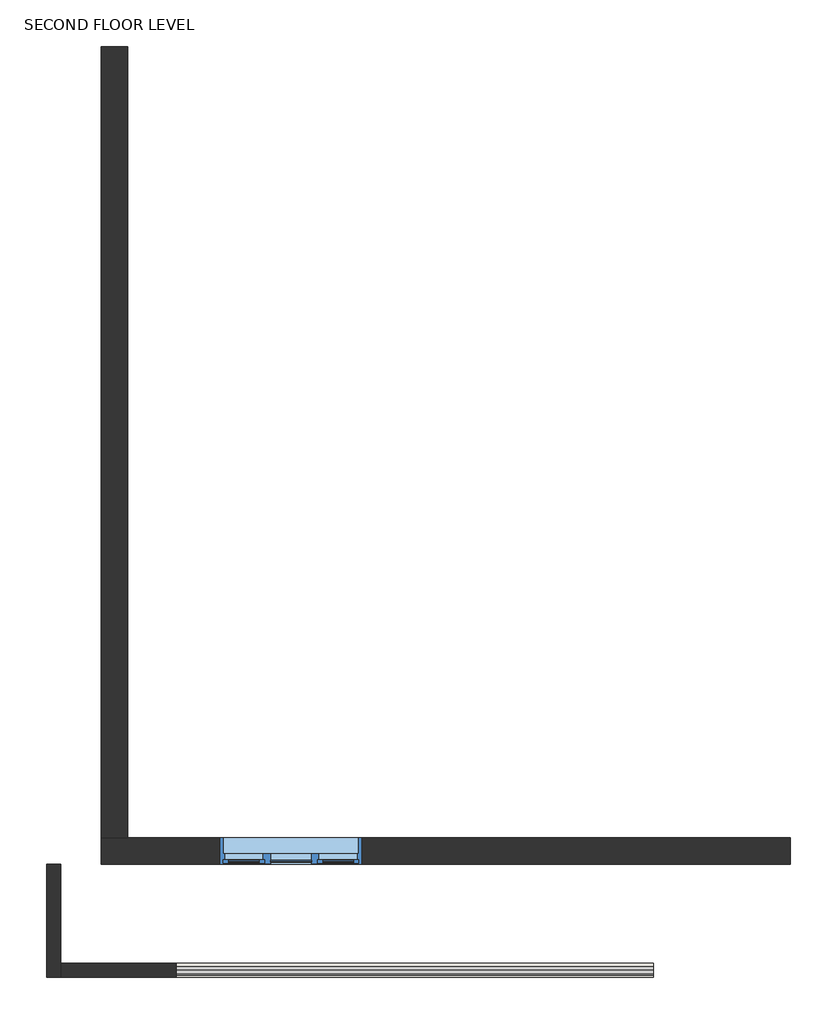
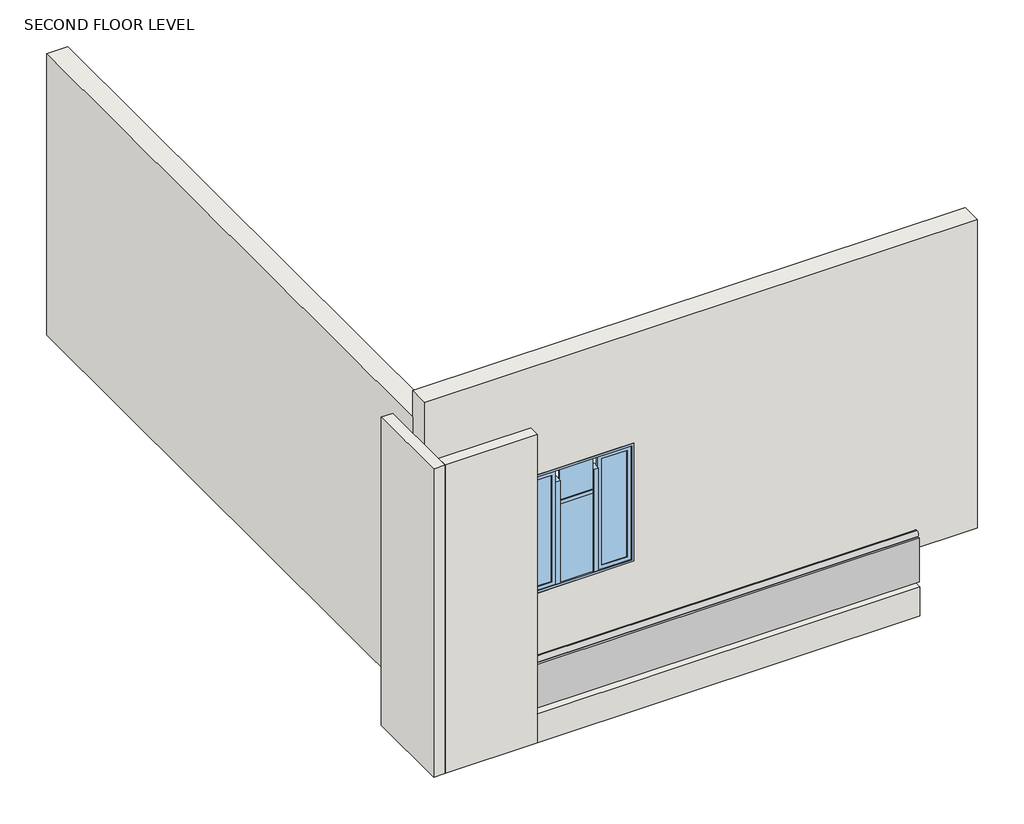
# One storey, incomplete: 5 walls, 1 member, 1 plate, 1 window.
"""IFC4 building model written with IfcOpenShell, lengths in millimetres."""

from ifc_helpers import new_model, si_unit, frame, origin, place, context, project, spatial, polyline, outline, extrude, faceted_brep, transform, mapped, element, save
from components import member_62657261, system_panel_glazed_289ab79d, window_273a115f

model = new_model("IFC4")

# Units and contexts
model_context = context("Model", 3, world=origin())
ifc_project = project(units=[si_unit("LENGTHUNIT", "METRE", prefix="MILLI")], contexts=[model_context])

# Site, building, storey
site = spatial("IfcSite", under=ifc_project)
building = spatial("IfcBuilding", under=site)
storey = spatial("IfcBuildingStorey", under=building, Name="SECOND FLOOR LEVEL", Elevation=7924.8)

# Member
placement = place(None, origin())
member_shape = member_62657261(model_context)
element("IfcMember", 1, ObjectType="Circular Mullion : 2.5\" Circular", at=placement, inside=storey, context=model_context, shape_type="MappedRepresentation", body=[
    mapped(member_shape, transform((7881.4271331, -12888.5768494, 8864.6), x_axis=(0.0, 0.0, 1.0), y_axis=(0.0, -1.0, 0.0), z_axis=(1.0, 0.0, 0.0))),
])

# Plate
system_panel_glazed_shape = system_panel_glazed_289ab79d(model_context)
element("IfcPlate", 2, ObjectType="System Panel : Glazed", at=placement, inside=storey, context=model_context, shape_type="MappedRepresentation", body=[
    mapped(system_panel_glazed_shape, transform((5824.0271331, -12888.5768494, 8305.8), x_axis=(1.0, 0.0, 0.0), y_axis=(0.0, 1.0, 0.0), z_axis=(0.0, 0.0, 1.0))),
])

# Walls
element("IfcWall", 3, ObjectType="9\"", at=placement, inside=storey, context=model_context, shape_type="Brep", body=[
    faceted_brep([(3118.9271331, -11975.7643494, 7924.8), (9062.5271331, -11975.7643494, 7924.8), (9062.5271331, -11975.7643494, 11430.0), (3118.9271331, -11975.7643494, 11430.0), (4147.6271331, -11975.7643494, 10185.4), (5366.8271331, -11975.7643494, 10185.4), (5366.8271331, -11975.7643494, 8839.2), (4147.6271331, -11975.7643494, 8839.2), (3118.9271331, -11747.1643494, 7924.8), (3118.9271331, -11747.1643494, 11127.6170633), (3118.9271331, -11747.1643494, 11430.0), (9062.5271331, -11747.1643494, 11430.0), (9062.5271331, -11747.1643494, 7924.8), (3347.5271331, -11747.1643494, 7924.8), (4147.6271331, -11747.1643494, 10185.4), (4147.6271331, -11747.1643494, 8839.2), (5366.8271331, -11747.1643494, 8839.2), (5366.8271331, -11747.1643494, 10185.4)], [[[0, 1, 2, 3], [4, 5, 6, 7]], [[8, 9, 10, 11, 12, 13], [14, 15, 16, 17]], [[1, 0, 8, 13, 12]], [[2, 1, 12, 11]], [[3, 2, 11, 10]], [[15, 14, 4, 7]], [[16, 15, 7, 6]], [[17, 16, 6, 5]], [[14, 17, 5, 4]], [[0, 3, 10, 9, 8]]]),
])
element("IfcWall", 4, ObjectType="9\"", at=placement, inside=storey, context=model_context, shape_type="SweptSolid", body=[
    extrude(outline(polyline([(3347.5271331, -4927.2643494), (3347.5271331, -11747.1643494), (3118.9271331, -11747.1643494), (3118.9271331, -4927.2643494), (3347.5271331, -4927.2643494)])), frame((0.0, 0.0, 7924.8), z_axis=(0.0, 0.0, 1.0), x_axis=(1.0, 0.0, 0.0)), (0.0, 0.0, 1.0), 3202.8170633),
])
element("IfcWall", 5, ObjectType="Interior - 4 7/8\" Partition (1-hr)", at=placement, inside=storey, context=model_context, shape_type="SweptSolid", body=[
    extrude(outline(polyline([(3766.6271331, -12826.6643494), (7881.4271331, -12826.6643494), (7881.4271331, -12950.4893494), (3766.6271331, -12950.4893494), (3766.6271331, -12826.6643494)])), frame((0.0, 0.0, 7924.8), z_axis=(0.0, 0.0, 1.0), x_axis=(1.0, 0.0, 0.0)), (0.0, 0.0, 1.0), 330.2),
])
element("IfcWall", 6, ObjectType="Interior - 4 7/8\" Partition (1-hr)", at=placement, inside=storey, context=model_context, shape_type="Brep", body=[
    faceted_brep([(2649.0271331, -11975.7643494, 7924.8), (2649.0271331, -12950.4893494, 7924.8), (2649.0271331, -12950.4893494, 11430.0), (2649.0271331, -11975.7643494, 11430.0), (2772.8521331, -11975.7643494, 7924.8), (2772.8521331, -11975.7643494, 11430.0), (2772.8521331, -12826.6643494, 11430.0), (2772.8521331, -12950.4893494, 11430.0), (2772.8521331, -12950.4893494, 7924.8), (2772.8521331, -12826.6643494, 7924.8)], [[[0, 1, 2, 3]], [[4, 5, 6, 7, 8, 9]], [[1, 0, 4, 9, 8]], [[3, 2, 7, 6, 5]], [[0, 3, 5, 4]], [[2, 1, 8, 7]]]),
])
element("IfcWall", 7, ObjectType="Interior - 4 7/8\" Partition (1-hr)", at=placement, inside=storey, context=model_context, shape_type="Brep", body=[
    faceted_brep([(3766.6271331, -12826.6643494, 7924.8), (2772.8521331, -12826.6643494, 7924.8), (2772.8521331, -12826.6643494, 11430.0), (3766.6271331, -12826.6643494, 11430.0), (3766.6271331, -12826.6643494, 8255.0), (3766.6271331, -12950.4893494, 7924.8), (3766.6271331, -12950.4893494, 8255.0), (3766.6271331, -12950.4893494, 11430.0), (2772.8521331, -12950.4893494, 11430.0), (2772.8521331, -12950.4893494, 7924.8)], [[[0, 1, 2, 3, 4]], [[5, 6, 7, 8, 9]], [[1, 0, 5, 9]], [[3, 2, 8, 7]], [[0, 4, 3, 7, 6, 5]], [[2, 1, 9, 8]]]),
])

# Window
window_shape = window_273a115f(model_context)
element("IfcWindow", 8, ObjectType="Window-Casement-Triple-Middle-Transom : 48\" x 53\"", at=placement, inside=storey, context=model_context, shape_type="MappedRepresentation", body=[
    mapped(window_shape, transform((4757.2271331, -11861.4643494, 7924.8), x_axis=(-1.0, 0.0, 0.0), y_axis=(0.0, -1.0, 0.0), z_axis=(0.0, 0.0, 1.0))),
])

save(model, "model.ifc")

# Revit data of these elements
# Type "Circular Mullion : 2.5\" Circular"
#   built-in parameter 1007350 = 0.104167 (stored number, unit not read)
# Type "System Panel : Glazed"
#   Construction Type Id = "GSP4R"
#   Analytic Construction = "1/8 in Pilkington single glazing"
#   Visual Light Transmittance = 0.9
#   Solar Heat Gain Coefficient = 0.86
#   Heat Transfer Coefficient (U) = 1.18115 BTU/(h·ft²·°F)
#   Define Thermal Properties by = 1
# Type "9\""
#   Assembly Code = "B2010"
#   Layers, outside or top first: 0' - 9" no material (function 1)
# Type "Interior - 4 7/8\" Partition (1-hr)"
#   Assembly Code = "C1010145"
#   Layers, outside or top first: 0' - 0 5/8" "Gypsum Wall Board" (function 5); 0' - 3 5/8" "Metal Stud Layer" (function 1); 0' - 0 5/8" "Gypsum Wall Board" (function 5)
# Type "Window-Casement-Triple-Middle-Transom : 48\" x 53\""
#   Type Mark = "18"
#   Fire Rating = "0.5h"
#   Assembly Code = "B2020100"
#   Analytic Construction = "Double glazing - domestic"
#   Window Width = 1' - 4"
#   Window Inset [instance default] = 0' - 0 5/8"
#   Wall Thickness [instance default] = 0' - 6"
#   Visual Light Transmittance = 0.81
#   Transom Height Ratio = 0.3
#   Thermal Resistance (R) = 1.8146 (h·ft²·°F)/BTU
#   Solar Heat Gain Coefficient = 0.76
#   Rough Width = 4' - 0 1/2"
#   Rough Height = 4' - 5 1/2"
#   Heat Transfer Coefficient (U) = 0.5511 BTU/(h·ft²·°F)
#   Height = 4' - 5"
#   Transom Height = 1' - 3.9"
#   Frame Gap 3 [instance default] = 0' - 1 83/128"
#   Frame Gap 2 [instance default] = 0' - 0 5/8"
#   Frame Gap 1 = 0' - 1 51/128"
#   Default Sill Height = 3' - 0"
#   Width = 4' - 0"
#   Frame Material = Metal - Aluminum
#   Glass Panel Material = Glass
#   Wall Closure = (empty or 0)
# Element 1 (IfcMember, "Circular Mullion : 2.5\" Circular")
#   Phase Created = New Construction
#   Materials on its faces: "Aluminum"
# Element 2 (IfcPlate, "System Panel : Glazed")
#   Phase Created = New Construction
#   Materials on its faces: "Glass"
# Element 3 (IfcWall, "9\"")
#   Top Offset = 0' - 0"
#   Base Offset = 0' - 0"
#   wall height = 11' - 6"
#   Phase Created = New Construction
#   Base Constraint = SECOND FLOOR LEVEL
#   Top Constraint = ROOF LEVEL
#   Materials on its faces: "Default Wall"
# Element 4 (IfcWall, "9\"")
#   Top Offset = 0' - 0"
#   Base Offset = 0' - 0"
#   Unconnected Height = 10' - 6.09516"
#   wall height = 10' - 6.09516"
#   Phase Created = New Construction
#   Base Constraint = SECOND FLOOR LEVEL
#   Materials on its faces: "Default Wall"
# Element 5 (IfcWall, "Interior - 4 7/8\" Partition (1-hr)")
#   Top Offset = 0' - 0"
#   Base Offset = 0' - 0"
#   Unconnected Height = 1' - 1"
#   wall height = 1' - 1"
#   Phase Created = New Construction
#   Base Constraint = SECOND FLOOR LEVEL
#   Materials on its faces: "Default Wall", "Gypsum Wall Board"
# Element 6 (IfcWall, "Interior - 4 7/8\" Partition (1-hr)")
#   Top Offset = 0' - 0"
#   Base Offset = 0' - 0"
#   wall height = 11' - 6"
#   Phase Created = New Construction
#   Base Constraint = SECOND FLOOR LEVEL
#   Top Constraint = ROOF LEVEL
#   Materials on its faces: "Gypsum Wall Board", "Default Wall"
# Element 7 (IfcWall, "Interior - 4 7/8\" Partition (1-hr)")
#   Top Offset = 0' - 0"
#   Base Offset = 0' - 0"
#   wall height = 11' - 6"
#   Phase Created = New Construction
#   Base Constraint = SECOND FLOOR LEVEL
#   Top Constraint = ROOF LEVEL
#   Materials on its faces: "Default Wall", "Gypsum Wall Board"
# Element 8 (IfcWindow, "Window-Casement-Triple-Middle-Transom : 48\" x 53\"")
#   Mark = "5"
#   Window Inset = 0' - 0 5/8"
#   Frame Gap 3 = 0' - 1 83/128"
#   Frame Gap 2 = 0' - 0 5/8"
#   Phase Created = New Construction
#   Materials on its faces: "Metal - Aluminum", "Glass"
# Materials
#   "Gypsum Wall Board": class "Generic", colour RGB 228 228 228, transparency 0, Description = "Gypsum Wall Board", Cost = 0
#   "Metal Stud Layer": class "Metal", colour RGB 199 199 199, transparency 0, Description = "Light gauge steel framing, thermal air layer", Cost = 0
#   "Metal - Aluminum": class "Metal", colour RGB 247 247 247, transparency 0
#   "Glass": class "Glass", colour RGB 0 128 192, transparency 0.75, Description = "Soda Lime Glass", Cost = 0
#   "Aluminum": class "Metal", colour RGB 247 247 247, transparency 0, Description = "Aluminum 6061", Cost = 0
#   "Default Wall": colour RGB 128 128 128, transparency 0, Cost = 0
